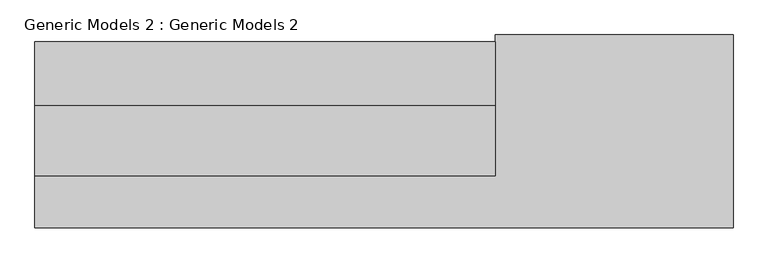
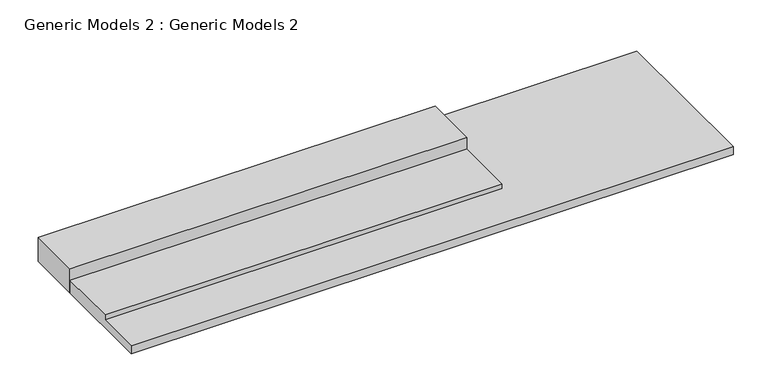
"""IFC4 building model written with IfcOpenShell, lengths in millimetres: proxy geometry, Generic Models 2 : Generic Models 2."""

from ifc_helpers import new_model, si_unit, origin, origin_with_axes, place, context, project, spatial, polyline, outline, extrude, faceted_brep, source, transform, mapped, element, save


def generic_models_2_generic_models_2_c2d7a446(model_context):
    return source(origin(), model_context, "Body", "SolidModel", [
        faceted_brep([(-15845.5386697, -13454.2956142, 66.2941501), (-15845.5386697, -13454.2956142, 0.0), (-11164.2034433, -13454.2956142, 0.0), (-11164.2034433, -13454.2956142, 66.2941501), (-15845.5386697, -13104.0774332, 66.2941501), (-15845.5386697, -13104.0774332, 105.1160061), (-15845.5386697, -12632.0114348, 105.1160061), (-15845.5386697, -12632.0114348, 0.0), (-12759.4386697, -12632.0114348, 0.0), (-12759.4386697, -12159.6557616, 0.0), (-11164.2034433, -12159.6557616, 0.0), (-11164.2034433, -12159.6557616, 66.2941501), (-12759.4386697, -12159.6557616, 66.2941501), (-12759.4386697, -12632.0114348, 66.2941501), (-12759.4386697, -13104.0774332, 66.2941501), (-12759.4386697, -13104.0774332, 105.1160061), (-12759.4386697, -12632.0114348, 105.1160061)], [[[0, 1, 2, 3]], [[1, 0, 4, 5, 6, 7]], [[1, 7, 8, 9, 10, 2]], [[4, 0, 3, 11, 12, 13, 14]], [[2, 10, 11, 3]], [[12, 9, 8, 13]], [[11, 10, 9, 12]], [[15, 5, 4, 14]], [[6, 16, 13, 8, 7]], [[16, 15, 14, 13]], [[5, 15, 16, 6]]]),
        extrude(outline(polyline([(-12759.4386697, -12632.0114348), (-15845.5386697, -12632.0114348), (-15845.5386697, -12204.6511954), (-12759.4386697, -12204.6511954), (-12759.4386697, -12632.0114348)])), origin_with_axes(), (0.0, 0.0, 1.0), 199.9236859),
    ])


if __name__ == "__main__":
    model = new_model("IFC4")
    model_context = context("Model", 3, world=origin())
    ifc_project = project(units=[si_unit("LENGTHUNIT", "METRE", prefix="MILLI")], contexts=[model_context])
    site = spatial("IfcSite", under=ifc_project)
    building = spatial("IfcBuilding", under=site)
    placement = place(None, origin())
    generic_models_2_generic_models_2_shape = generic_models_2_generic_models_2_c2d7a446(model_context)
    element("IfcBuildingElementProxy", 1, Name="Generic Models 2 : Generic Models 2", ObjectType="Generic Models 2 : Generic Models 2", at=placement, inside=building, context=model_context, shape_type="MappedRepresentation", body=[
        mapped(generic_models_2_generic_models_2_shape, transform((0.0, 0.0, 0.0), x_axis=(1.0, 0.0, 0.0), y_axis=(0.0, 1.0, 0.0), z_axis=(0.0, 0.0, 1.0))),
    ])
    save(model, "model.ifc")
